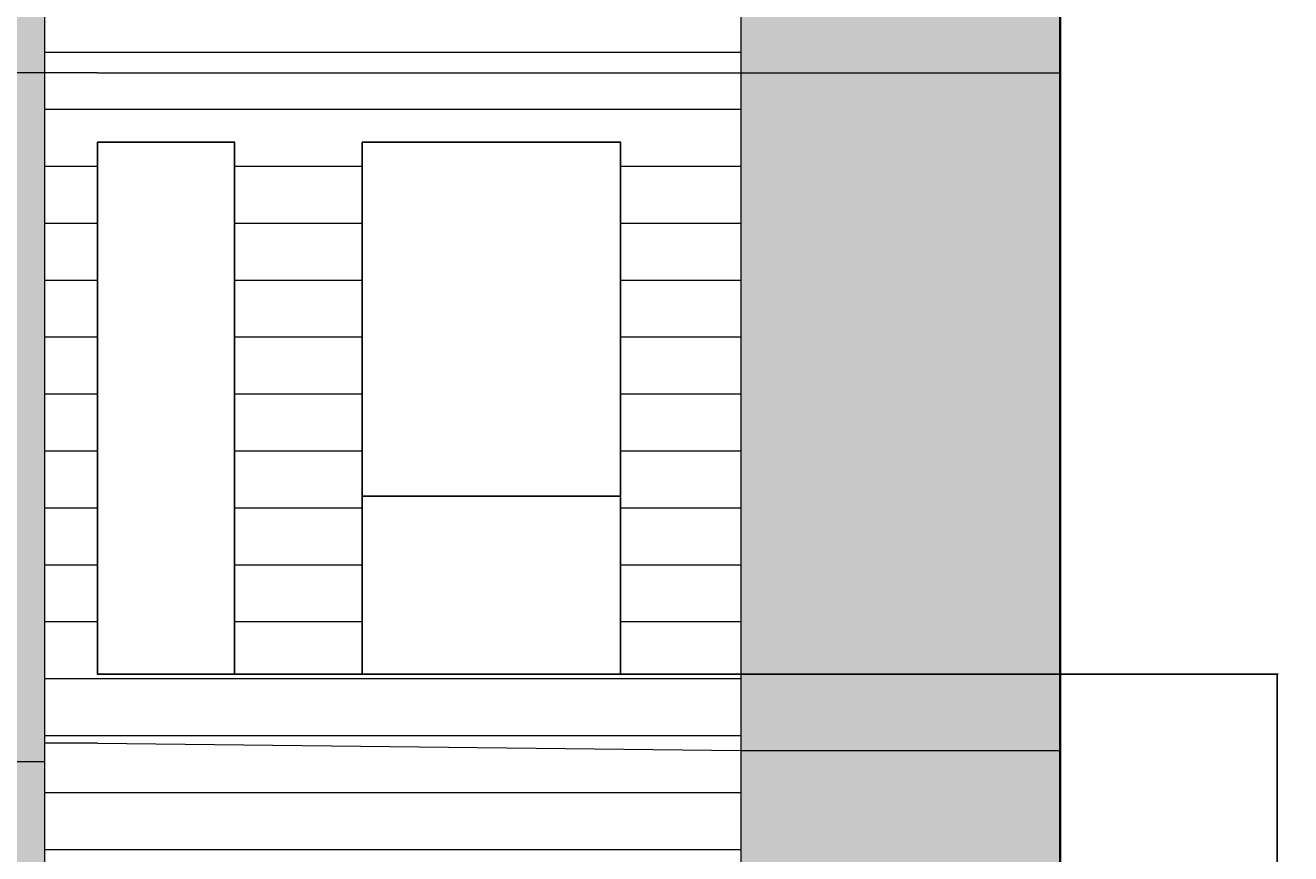
# Model space of a CAD drawing. Units: inches. Extents: x 8 to 634, y 41 to 867.
# Tile 13 of 21: x 415 to 634, y 434 to 577. Entities that reach past the tile are written whole.
import ezdxf

# ---------------------------------------------------------------- set-up
doc = ezdxf.new("R2010")
doc.units = ezdxf.units.IN
doc.header["$MEASUREMENT"] = 0
for name, color, linetype, lineweight in [('A-ANNO-DIMS', 2, 'Continuous', 18), ('A-GLAZ', 4, 'Continuous', 25), ('A-WALL', 7, 'Continuous', 35), ('A-WALL-PANL', 7, 'Continuous', 18), ('A-WALL-PATT', 8, 'Continuous', 9)]:
    doc.layers.add(name, color=color, linetype=linetype, lineweight=lineweight)
doc.styles.get("Standard").update_dxf_attribs({"font": 'arial.ttf'})
doc.dimstyles.get("Standard").update_dxf_attribs({"dimtxt": 1.125, "dimasz": 0.18, "dimexe": 0.18, "dimexo": 0.0625, "dimgap": 0.09, "dimtad": 0, "dimtih": 1, "dimtoh": 1, "dimdec": 4, "dimzin": 0, "dimdsep": 46, "dimlunit": 4, "dimtxsty": 'Standard', "dimcen": 0.09, "dimadec": 0, "dimazin": 0, "dimtfac": 1, "dimtdec": 4, "dimtofl": 0, "dimtmove": 0, "dimatfit": 3, "dimfxl": 1, "dimtolj": 1, "dimtzin": 0, "dimarcsym": 0})

# ---------------------------------------------------------------- blocks, each defined once
blk = doc.blocks.new('WIN-NARROW-FIXED')
blk.add_lwpolyline([(0, 92.26), (23.77, 92.26), (23.77, 0), (0, 0)], close=True)
blk = doc.blocks.new('WIN-WIDE-TRANSOM')
blk.add_line((0, 30.85), (44.78, 30.85))
blk.add_lwpolyline([(0, 92.26), (44.78, 92.26), (44.78, 0), (0, 0)], close=True)
blk = doc.blocks.new('*D40')
at = {"layer": 'A-ANNO-DIMS', "color": 0, "lineweight": -2, "transparency": 16777216}
for p, q in [((427.5, 464.91), (632.18, 464.91)), ((632, 464.73), (632, 377.2)), ((632, 288.35), (632, 375.87)), ((427.5, 288.17), (632.18, 288.17))]:
    blk.add_line(p, q, dxfattribs=at)
at = {"layer": 'A-ANNO-DIMS', "color": 0, "transparency": 16777216}
for points in [[(631.97, 464.73), (632.03, 464.73), (632, 464.91)], [(631.97, 288.35), (632.03, 288.35), (632, 288.17)]]:
    blk.add_solid(points, dxfattribs=at)
at = {"layer": 'Defpoints', "color": 0, "transparency": 16777216}
for p in [(427.44, 464.91), (632, 464.91), (427.44, 288.17)]:
    blk.add_point(p, dxfattribs=at)
at = {"layer": 'A-ANNO-DIMS', "color": 0, "transparency": 16777216, "insert": (632, 376.54), "char_height": 1.125, "attachment_point": 5}
blk.add_mtext('\\A1;176.74', dxfattribs=at)

msp = doc.modelspace()

# ---------------------------------------------------------------- hatches: boundary and pattern name
at = {"layer": 'A-WALL-PATT', "transparency": 33554687}
h = msp.add_hatch(dxfattribs=at)
h.set_pattern_fill('ANSI31', color=256, scale=79, angle=135)
h.paths.add_polyline_path([(539.0002, 276.166), (499.4677, 276.166), (418.2881, 276.166), (418.2881, 228.4951), (435.5682, 228.4951), (539.0002, 228.4951)])
h.paths.add_polyline_path([(539.0002, 228.4951), (435.5682, 228.4951), (418.2881, 228.4951), (418.2881, 112.2342), (439.3242, 112.2342), (539.0002, 112.2342)])
h.paths.add_polyline_path([(518.1129, 124.2342), (473.3277, 124.2342), (473.3277, 216.4951), (518.1129, 216.4951)], flags=16)
h.paths.add_polyline_path([(451.2116, 124.2342), (427.4368, 124.2342), (427.4368, 216.4951), (451.2116, 216.4951)], flags=16)
h.paths.add_polyline_path([(539.0002, 112.2342), (439.3242, 112.2342), (418.2881, 112.2342), (418.2881, 91.5417), (539.0002, 91.5417)])
h.paths.add_polyline_path([(539.0002, 392.4268), (427.4368, 392.4268), (418.2881, 392.4268), (418.2881, 391.7598), (418.2881, 276.166), (499.4677, 276.166), (539.0002, 276.166)])
h.paths.add_polyline_path([(518.1129, 288.166), (473.3277, 288.166), (473.3277, 380.4268), (518.1129, 380.4268)], flags=16)
h.paths.add_polyline_path([(451.2116, 288.166), (427.4368, 288.166), (427.4368, 380.4268), (451.2116, 380.4268)], flags=16)
h.paths.add_polyline_path([(539.0002, 451.6305), (427.4368, 452.9097), (418.2881, 452.9097), (418.2881, 392.4268), (427.4368, 392.4268), (539.0002, 392.4268)])
h.paths.add_polyline_path([(539.0002, 569.1705), (427.4368, 569.1705), (418.2881, 569.1705), (418.2881, 452.9097), (427.4368, 452.9097), (539.0002, 451.6305)])
h.paths.add_polyline_path([(473.3277, 557.1705), (518.1129, 557.1705), (518.1129, 464.9097), (473.3277, 464.9097)], flags=16)
h.paths.add_polyline_path([(451.2116, 557.1705), (451.2116, 464.9097), (427.4368, 464.9097), (427.4368, 557.1705)], flags=16)
h.paths.add_polyline_path([(539.0002, 619.6298), (418.2881, 619.6298), (418.2881, 569.1705), (427.4368, 569.1705), (539.0002, 569.1705)])
h.paths.add_polyline_path([(556.7072, 774.3342), (556.7072, 776.8929), (299.7961, 776.8929), (299.7961, 697.6655), (322.56, 697.6655), (322.56, 740.5561), (355.7466, 740.5561), (355.7466, 697.6655), (360.785, 697.6655), (370.3877, 697.6655), (370.3877, 740.5561), (439.201, 740.5561), (439.201, 691.978), (449.4498, 691.978), (449.4498, 740.5561), (498.2535, 740.5561), (498.2535, 691.978), (508.5023, 691.978), (508.5023, 740.5561), (536.3204, 740.5561), (536.3204, 691.978), (539.0002, 691.978), (539.0002, 697.6655), (556.7072, 697.6655)])
h = msp.add_hatch(dxfattribs=at)
h.set_pattern_fill('AR-CONC', color=256, scale=3.2)
h.paths.add_polyline_path([(119.7065, 697.6655), (47.3401, 697.6655), (47.3401, 569.1705), (119.7065, 569.1705)])
h.paths.add_polyline_path([(202.1558, 697.6655), (119.7065, 697.6655), (119.7065, 569.1705), (202.1558, 569.1705)])
h.paths.add_polyline_path([(284.6051, 697.6655), (202.1558, 697.6655), (202.1558, 569.1705), (284.6051, 569.1705)])
h.paths.add_polyline_path([(119.7065, 569.1705), (47.3401, 569.1705), (47.3401, 523.5555), (47.3401, 449.7533), (119.7065, 449.7533)])
h.paths.add_polyline_path([(342.6544, 682.1444), (360.785, 697.6655), (284.6051, 697.6655), (284.6051, 569.1705), (342.6544, 569.1705)])
h.paths.add_polyline_path([(342.6544, 569.1705), (284.6051, 569.1705), (284.6051, 449.7533), (342.6544, 449.7533)])
h.paths.add_polyline_path([(418.2881, 691.978), (418.2881, 697.6655), (360.785, 697.6655), (360.785, 569.1705), (418.2881, 569.1705)])
h.paths.add_polyline_path([(418.2881, 569.1705), (360.785, 569.1705), (360.785, 523.5555), (360.785, 449.7533), (418.2881, 449.7533)])
h.paths.add_polyline_path([(594.3501, 697.6655), (539.0002, 697.6655), (539.0002, 691.978), (539.0002, 569.1705), (594.3501, 569.1705)])
h.paths.add_polyline_path([(594.3501, 523.5555), (594.3501, 569.1705), (539.0002, 569.1705), (539.0002, 451.6305), (594.3501, 451.6305)])
h.paths.add_polyline_path([(594.3501, 451.6305), (539.0002, 451.6305), (539.0002, 391.7598), (594.3501, 391.7598)])
h.paths.add_polyline_path([(594.3501, 391.7598), (539.0002, 391.7598), (539.0002, 276.166), (594.3501, 276.166)])
h.paths.add_polyline_path([(418.2881, 449.7533), (360.785, 449.7533), (360.785, 391.7598), (418.2881, 391.7598)])
h.paths.add_polyline_path([(342.6544, 449.7533), (284.6051, 449.7533), (284.6051, 391.7598), (342.6544, 391.7598)])
h.paths.add_polyline_path([(342.6544, 391.7598), (284.6051, 391.7598), (284.6051, 272.3426), (342.6544, 272.3426)])
h.paths.add_polyline_path([(418.2881, 391.7598), (360.785, 391.7598), (360.785, 272.3426), (418.2881, 272.3426)])
h.paths.add_polyline_path([(418.2881, 272.3426), (360.785, 272.3426), (360.785, 235.5555), (418.2881, 235.5555)])
h.paths.add_polyline_path([(342.6544, 272.3426), (284.6051, 272.3426), (284.6051, 235.5555), (295.0049, 235.5555), (342.6544, 235.5555)])
h.paths.add_polyline_path([(594.3501, 276.166), (539.0002, 276.166), (539.0002, 228.4951), (594.3501, 228.4951)])
h.paths.add_polyline_path([(594.3501, 228.4951), (539.0002, 228.4951), (539.0002, 91.5417), (594.3501, 91.5417)])
h.paths.add_polyline_path([(418.2881, 235.5555), (360.785, 235.5555), (360.785, 91.5417), (418.2881, 91.5417)])
h.paths.add_polyline_path([(284.6051, 272.3426), (119.7065, 272.3426), (119.7065, 235.5555), (284.6051, 235.5555)])
h.paths.add_polyline_path([(119.7065, 272.3426), (47.3401, 272.3426), (47.3401, 235.5555), (47.3401, 91.5555), (63.5448, 91.5555), (63.5448, 227.8036), (268.998, 227.8036), (268.998, 91.5555), (295.0049, 91.5555), (295.0049, 222.583), (271.9787, 222.583), (271.9787, 229.0481), (62.4019, 229.0481), (62.4019, 222.583), (61.1827, 222.583), (61.1827, 235.5555), (119.7065, 235.5555)])
h.paths.add_polyline_path([(119.7065, 391.7598), (47.3401, 391.7598), (47.3401, 379.5555), (47.3401, 272.3426), (119.7065, 272.3426)])
h.paths.add_polyline_path([(119.7065, 449.7533), (47.3401, 449.7533), (47.3401, 391.7598), (119.7065, 391.7598)])
h.paths.add_polyline_path([(202.1558, 449.7533), (119.7065, 449.7533), (119.7065, 391.7598), (202.1558, 391.7598)])
h.paths.add_polyline_path([(284.6051, 449.7533), (202.1558, 449.7533), (202.1558, 391.7598), (284.6051, 391.7598)])

# ---------------------------------------------------------------- linework, layer by layer
at = {"layer": 'A-WALL'}
for p, q in [((594.3501, 523.5555), (594.3501, 697.6655)), ((594.3501, 91.5417), (594.3501, 523.5555))]:
    msp.add_line(p, q, dxfattribs=at)
at = {"layer": 'A-WALL-PANL'}
for p, q in [((418.2881, 569.1705), (47.3401, 569.1705)), ((427.4368, 569.1705), (418.2881, 569.1705)), ((427.4368, 569.1705), (539.0002, 569.1705)), ((539.0002, 569.1705), (594.3501, 569.1705)), ((427.4368, 452.9097), (418.2881, 452.9097)), ((427.4368, 452.9097), (539.0002, 451.6305)), ((539.0002, 451.6305), (594.3501, 451.6305)), ((284.6051, 449.7533), (418.2881, 449.7533))]:
    msp.add_line(p, q, dxfattribs=at)
msp.add_lwpolyline([(539.0002, 691.978), (539.0002, 91.5417), (418.2881, 91.5417), (418.2881, 691.978)], dxfattribs=at)

# ---------------------------------------------------------------- block references
at = {"layer": 'A-GLAZ'}
for name, p in [('WIN-NARROW-FIXED', (427.437, 464.9095)), ('WIN-WIDE-TRANSOM', (473.328, 464.9095))]:
    msp.add_blockref(name, p, dxfattribs=at)

# ---------------------------------------------------------------- dimensions: what is measured, and where the dimension line sits
at = {"layer": 'A-ANNO-DIMS'}
dim = msp.add_linear_dim(base=(632.0001, 464.9097), p1=(427.4368, 288.166), p2=(427.4368, 464.9097), angle=90, dimstyle='Standard', override={"dimdec": 2, "dimlfac": 1, "dimrnd": 0, "dimzin": 0, "dimdsep": 46, "dimlunit": 2}, dxfattribs=at)
dim.commit()
dim.dimension.update_dxf_attribs({"geometry": '*D40', "text_midpoint": (632.0001, 376.5379)})

doc.saveas('drawing.dxf')
